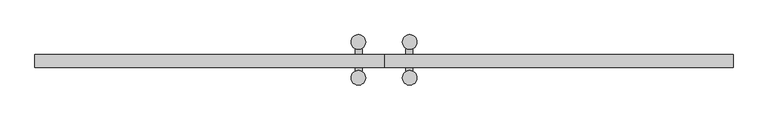
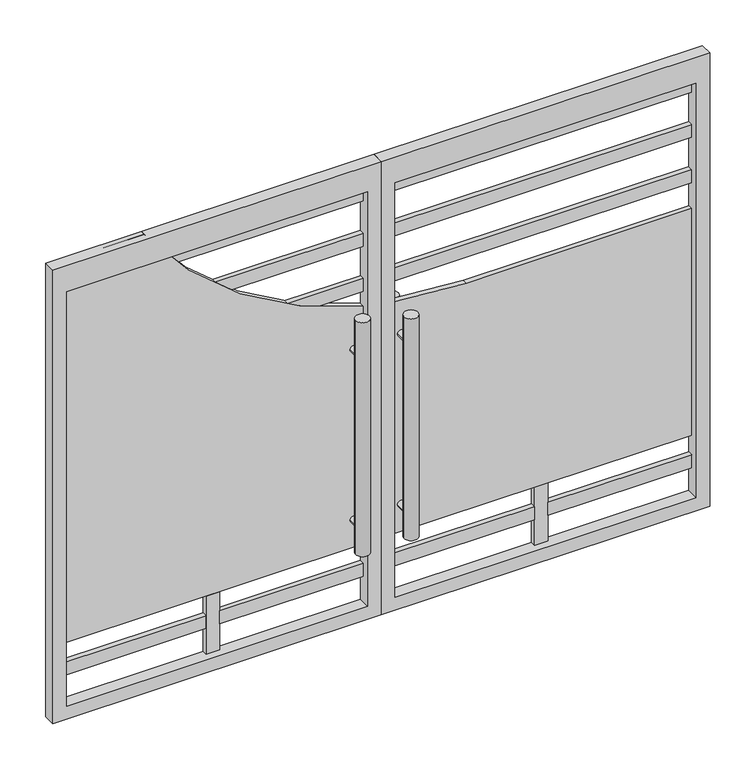
"""IFC4 building model written with IfcOpenShell, lengths in millimetres: proxy geometry."""

from ifc_helpers import new_model, si_unit, point, frame, frame_2d, origin, place, context, project, spatial, polyline, circle_curve, trimmed, segment, composite_curve, outline, extrude, source, transform, mapped, element, save


def generic_models_9a79fa98(model_context):
    return source(origin(), model_context, "Body", "SweptSolid", [
        extrude(outline(polyline([(0.0, -1219.2), (0.0, 0.0), (1778.0, 0.0), (1778.0, -1219.2), (0.0, -1219.2)]), holes=[polyline([(50.8, -1168.4), (1676.4, -1168.4), (1676.4, -50.8), (50.8, -50.8), (50.8, -1168.4)])]), frame((0.0, -46.0617726, 0.0), z_axis=(0.0, 1.0, 0.0), x_axis=(0.0, 0.0, 1.0)), (0.0, 0.0, 1.0), 46.0617726),
        extrude(outline(polyline([(0.0, 1219.2), (1778.0, 1219.2), (1778.0, 0.0), (0.0, 0.0), (0.0, 1219.2)]), holes=[polyline([(50.8, 1168.4), (50.8, 50.8), (1676.4, 50.8), (1676.4, 1168.4), (50.8, 1168.4)])]), frame((0.0, -46.0617726, 0.0), z_axis=(0.0, 1.0, 0.0), x_axis=(0.0, 0.0, 1.0)), (0.0, 0.0, 1.0), 46.0617726),
        extrude(outline(composite_curve([segment(polyline([(1778.0, -1168.4), (279.4, -1168.4), (279.4, -50.8), (1212.1744192, -50.8)]), True, "CONTINUOUS"), segment(trimmed(circle_curve(frame_2d((2582.6324877, 299.8877691)), 1414.6155764), [point((1212.1744192, -50.8))], [point((1778.0, -863.6))], True, "CARTESIAN"), True, "CONTINUOUS"), segment(polyline([(1778.0, -863.6), (1778.0, -1168.4)]), True, "CONTINUOUS")], self_intersect=False)), frame((0.0, -19.05, 0.0), z_axis=(0.0, 1.0, 0.0), x_axis=(0.0, 0.0, 1.0)), (0.0, 0.0, 1.0), 19.05),
        extrude(outline(composite_curve([segment(polyline([(279.4, 1168.4), (1168.4, 1168.4), (1168.4, 332.8073642)]), True, "CONTINUOUS"), segment(trimmed(circle_curve(frame_2d((2582.6324877, 299.8877691)), 1414.6155764), [point((1168.4, 332.8073642))], [point((1190.1194672, 50.8))], True, "CARTESIAN"), True, "CONTINUOUS"), segment(polyline([(1190.1194672, 50.8), (279.4, 50.8), (279.4, 1168.4)]), True, "CONTINUOUS")], self_intersect=False)), frame((0.0, -19.05, 0.0), z_axis=(0.0, 1.0, 0.0), x_axis=(0.0, 0.0, 1.0)), (0.0, 0.0, 1.0), 19.05),
        extrude(outline(composite_curve([segment(polyline([(1676.4, -50.8), (1676.4, -786.3350015)]), True, "CONTINUOUS"), segment(trimmed(circle_curve(frame_2d((2582.6324877, 299.8877691)), 1414.6155764), [point((1676.4, -786.3350015))], [point((1625.6, -741.8540639))], False, "CARTESIAN"), True, "CONTINUOUS"), segment(polyline([(1625.6, -741.8540639), (1625.6, -50.8), (1676.4, -50.8)]), True, "CONTINUOUS")], self_intersect=False)), frame((0.0, -19.05, 0.0), z_axis=(0.0, 1.0, 0.0), x_axis=(0.0, 0.0, 1.0)), (0.0, 0.0, 1.0), 19.05),
        extrude(outline(polyline([(1171.575, -19.05), (50.8, -19.05), (50.8, 0.0), (1171.575, 0.0), (1171.575, -19.05)])), frame((0.0, 0.0, 1625.6), z_axis=(0.0, 0.0, 1.0), x_axis=(1.0, 0.0, 0.0)), (0.0, 0.0, 1.0), 50.8),
        extrude(outline(composite_curve([segment(polyline([(1498.6, -50.8), (1498.6, -608.963591)]), True, "CONTINUOUS"), segment(trimmed(circle_curve(frame_2d((2582.6324877, 299.8877691)), 1414.6155764), [point((1498.6, -608.963591))], [point((1447.8, -544.6786605))], False, "CARTESIAN"), True, "CONTINUOUS"), segment(polyline([(1447.8, -544.6786605), (1447.8, -50.8), (1498.6, -50.8)]), True, "CONTINUOUS")], self_intersect=False)), frame((0.0, -19.05, 0.0), z_axis=(0.0, 1.0, 0.0), x_axis=(0.0, 0.0, 1.0)), (0.0, 0.0, 1.0), 19.05),
        extrude(outline(polyline([(1171.575, -19.05), (50.8, -19.05), (50.8, 0.0), (1171.575, 0.0), (1171.575, -19.05)])), frame((0.0, 0.0, 1447.8), z_axis=(0.0, 0.0, 1.0), x_axis=(1.0, 0.0, 0.0)), (0.0, 0.0, 1.0), 50.8),
        extrude(outline(composite_curve([segment(polyline([(1320.8, -50.8), (1320.8, -339.5776342)]), True, "CONTINUOUS"), segment(trimmed(circle_curve(frame_2d((2582.6324877, 299.8877691)), 1414.6155764), [point((1320.8, -339.5776342))], [point((1270.0, -227.4955652))], False, "CARTESIAN"), True, "CONTINUOUS"), segment(polyline([(1270.0, -227.4955652), (1270.0, -50.8), (1320.8, -50.8)]), True, "CONTINUOUS")], self_intersect=False)), frame((0.0, -19.05, 0.0), z_axis=(0.0, 1.0, 0.0), x_axis=(0.0, 0.0, 1.0)), (0.0, 0.0, 1.0), 19.05),
        extrude(outline(polyline([(1171.575, -19.05), (50.8, -19.05), (50.8, 0.0), (1171.575, 0.0), (1171.575, -19.05)])), frame((0.0, 0.0, 1270.0), z_axis=(0.0, 0.0, 1.0), x_axis=(1.0, 0.0, 0.0)), (0.0, 0.0, 1.0), 50.8),
        extrude(outline(polyline([(-635.0, -19.05), (-1168.4, -19.05), (-1168.4, 0.0), (-635.0, 0.0), (-635.0, -19.05)])), frame((0.0, 0.0, 152.4), z_axis=(0.0, 0.0, 1.0), x_axis=(1.0, 0.0, 0.0)), (0.0, 0.0, 1.0), 50.8),
        extrude(outline(polyline([(-50.8, -19.05), (-584.2, -19.05), (-584.2, 0.0), (-50.8, 0.0), (-50.8, -19.05)])), frame((0.0, 0.0, 152.4), z_axis=(0.0, 0.0, 1.0), x_axis=(1.0, 0.0, 0.0)), (0.0, 0.0, 1.0), 50.8),
        extrude(outline(polyline([(1168.4, -19.05), (635.0, -19.05), (635.0, 0.0), (1168.4, 0.0), (1168.4, -19.05)])), frame((0.0, 0.0, 152.4), z_axis=(0.0, 0.0, 1.0), x_axis=(1.0, 0.0, 0.0)), (0.0, 0.0, 1.0), 50.8),
        extrude(outline(polyline([(584.2, -19.05), (50.8, -19.05), (50.8, 0.0), (584.2, 0.0), (584.2, -19.05)])), frame((0.0, 0.0, 152.4), z_axis=(0.0, 0.0, 1.0), x_axis=(1.0, 0.0, 0.0)), (0.0, 0.0, 1.0), 50.8),
        extrude(outline(polyline([(-584.2, -19.05), (-635.0, -19.05), (-635.0, 0.0), (-584.2, 0.0), (-584.2, -19.05)])), frame((0.0, 0.0, 50.8), z_axis=(0.0, 0.0, 1.0), x_axis=(1.0, 0.0, 0.0)), (0.0, 0.0, 1.0), 228.6),
        extrude(outline(polyline([(635.0, -19.05), (584.2, -19.05), (584.2, 0.0), (635.0, 0.0), (635.0, -19.05)])), frame((0.0, 0.0, 50.8), z_axis=(0.0, 0.0, 1.0), x_axis=(1.0, 0.0, 0.0)), (0.0, 0.0, 1.0), 228.6),
        extrude(outline(composite_curve([segment(trimmed(circle_curve(frame_2d((-89.7949058, 43.7785099)), 25.4), [point((-64.3949058, 43.7785099))], [point((-115.1949058, 43.7785099))], False, "CARTESIAN"), True, "CONTINUOUS"), segment(trimmed(circle_curve(frame_2d((-89.7949058, 43.7785099)), 25.4), [point((-115.1949058, 43.7785099))], [point((-64.3949058, 43.7785099))], False, "CARTESIAN"), True, "CONTINUOUS")], self_intersect=False)), frame((0.0, 0.0, 279.4), z_axis=(0.0, 0.0, 1.0), x_axis=(1.0, 0.0, 0.0)), (0.0, 0.0, 1.0), 889.0),
        extrude(outline(composite_curve([segment(trimmed(circle_curve(frame_2d((89.7949058, 43.7785099)), 25.4), [point((64.3949058, 43.7785099))], [point((115.1949058, 43.7785099))], False, "CARTESIAN"), True, "CONTINUOUS"), segment(trimmed(circle_curve(frame_2d((89.7949058, 43.7785099)), 25.4), [point((115.1949058, 43.7785099))], [point((64.3949058, 43.7785099))], False, "CARTESIAN"), True, "CONTINUOUS")], self_intersect=False)), frame((0.0, 0.0, 279.4), z_axis=(0.0, 0.0, 1.0), x_axis=(1.0, 0.0, 0.0)), (0.0, 0.0, 1.0), 889.0),
        extrude(outline(composite_curve([segment(trimmed(circle_curve(frame_2d((-89.7949058, -81.8785099)), 25.4), [point((-64.3949058, -81.8785099))], [point((-115.1949058, -81.8785099))], False, "CARTESIAN"), True, "CONTINUOUS"), segment(trimmed(circle_curve(frame_2d((-89.7949058, -81.8785099)), 25.4), [point((-115.1949058, -81.8785099))], [point((-64.3949058, -81.8785099))], False, "CARTESIAN"), True, "CONTINUOUS")], self_intersect=False)), frame((0.0, 0.0, 298.8472671), z_axis=(0.0, 0.0, 1.0), x_axis=(1.0, 0.0, 0.0)), (0.0, 0.0, 1.0), 917.3073645),
        extrude(outline(composite_curve([segment(trimmed(circle_curve(frame_2d((89.7949058, -81.8785099)), 25.4), [point((64.3949058, -81.8785099))], [point((115.1949058, -81.8785099))], False, "CARTESIAN"), True, "CONTINUOUS"), segment(trimmed(circle_curve(frame_2d((89.7949058, -81.8785099)), 25.4), [point((115.1949058, -81.8785099))], [point((64.3949058, -81.8785099))], False, "CARTESIAN"), True, "CONTINUOUS")], self_intersect=False)), frame((0.0, 0.0, 298.8472671), z_axis=(0.0, 0.0, 1.0), x_axis=(1.0, 0.0, 0.0)), (0.0, 0.0, 1.0), 869.5527329),
        extrude(outline(composite_curve([segment(trimmed(circle_curve(frame_2d((1058.3458504, 88.119132)), 12.7), [point((1058.3458504, 75.419132))], [point((1058.3458504, 100.819132))], False, "CARTESIAN"), True, "CONTINUOUS"), segment(trimmed(circle_curve(frame_2d((1058.3458504, 88.119132)), 12.7), [point((1058.3458504, 100.819132))], [point((1058.3458504, 75.419132))], False, "CARTESIAN"), True, "CONTINUOUS")], self_intersect=False)), frame((0.0, -57.15, 0.0), z_axis=(0.0, 1.0, 0.0), x_axis=(0.0, 0.0, 1.0)), (0.0, 0.0, 1.0), 76.6172039),
        extrude(outline(composite_curve([segment(trimmed(circle_curve(frame_2d((389.4541496, 88.119132)), 12.7), [point((389.4541496, 75.419132))], [point((389.4541496, 100.819132))], False, "CARTESIAN"), True, "CONTINUOUS"), segment(trimmed(circle_curve(frame_2d((389.4541496, 88.119132)), 12.7), [point((389.4541496, 100.819132))], [point((389.4541496, 75.419132))], False, "CARTESIAN"), True, "CONTINUOUS")], self_intersect=False)), frame((0.0, -57.15, 0.0), z_axis=(0.0, 1.0, 0.0), x_axis=(0.0, 0.0, 1.0)), (0.0, 0.0, 1.0), 76.7981605),
        extrude(outline(composite_curve([segment(trimmed(circle_curve(frame_2d((1058.3458504, -88.119132)), 12.7), [point((1058.3458504, -75.419132))], [point((1058.3458504, -100.819132))], False, "CARTESIAN"), True, "CONTINUOUS"), segment(trimmed(circle_curve(frame_2d((1058.3458504, -88.119132)), 12.7), [point((1058.3458504, -100.819132))], [point((1058.3458504, -75.419132))], False, "CARTESIAN"), True, "CONTINUOUS")], self_intersect=False)), frame((0.0, -57.15, 0.0), z_axis=(0.0, 1.0, 0.0), x_axis=(0.0, 0.0, 1.0)), (0.0, 0.0, 1.0), 76.6172039),
        extrude(outline(composite_curve([segment(trimmed(circle_curve(frame_2d((389.4541496, -88.119132)), 12.7), [point((389.4541496, -75.419132))], [point((389.4541496, -100.819132))], False, "CARTESIAN"), True, "CONTINUOUS"), segment(trimmed(circle_curve(frame_2d((389.4541496, -88.119132)), 12.7), [point((389.4541496, -100.819132))], [point((389.4541496, -75.419132))], False, "CARTESIAN"), True, "CONTINUOUS")], self_intersect=False)), frame((0.0, -57.15, 0.0), z_axis=(0.0, 1.0, 0.0), x_axis=(0.0, 0.0, 1.0)), (0.0, 0.0, 1.0), 76.7981605),
    ])


if __name__ == "__main__":
    model = new_model("IFC4")
    model_context = context("Model", 3, world=origin())
    ifc_project = project(units=[si_unit("LENGTHUNIT", "METRE", prefix="MILLI")], contexts=[model_context])
    site = spatial("IfcSite", under=ifc_project)
    building = spatial("IfcBuilding", under=site)
    placement = place(None, origin())
    generic_models_shape = generic_models_9a79fa98(model_context)
    element("IfcBuildingElementProxy", 1, Name="Generic Models", at=placement, inside=building, context=model_context, shape_type="MappedRepresentation", body=[
        mapped(generic_models_shape, transform((0.0, 0.0, 0.0), x_axis=(1.0, 0.0, 0.0), y_axis=(0.0, 1.0, 0.0), z_axis=(0.0, 0.0, 1.0))),
    ])
    save(model, "model.ifc")

# Revit data of these elements
# Type
#   sheet = none
#   pipe = none
#   handal = none
#   faram = none
#   Default Elevation = 0
